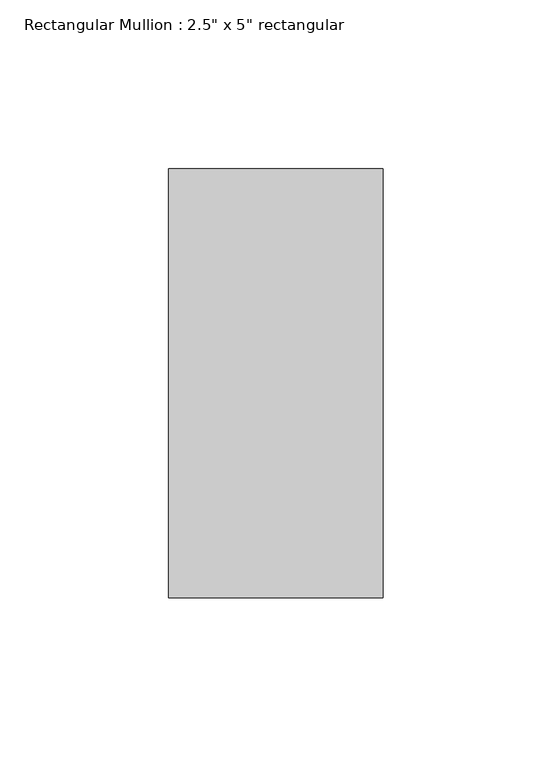
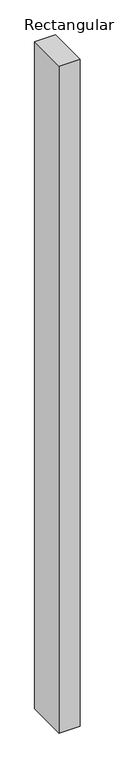
"""IFC4 building model written with IfcOpenShell, lengths in millimetres: member geometry."""

from ifc_helpers import new_model, si_unit, frame, origin, place, context, project, spatial, polyline, outline, extrude, source, transform, mapped, element, save


def member_cad56782(model_context):
    return source(origin(), model_context, "Body", "SweptSolid", [
        extrude(outline(polyline([(31.75, 63.5), (31.75, -63.5), (-31.75, -63.5), (-31.75, 63.5), (31.75, 63.5)])), frame((0.0, 0.0, -2129.1310998), z_axis=(0.0, 0.0, 1.0), x_axis=(1.0, 0.0, 0.0)), (0.0, 0.0, 1.0), 2129.1310998),
    ])


if __name__ == "__main__":
    model = new_model("IFC4")
    model_context = context("Model", 3, world=origin())
    ifc_project = project(units=[si_unit("LENGTHUNIT", "METRE", prefix="MILLI")], contexts=[model_context])
    site = spatial("IfcSite", under=ifc_project)
    building = spatial("IfcBuilding", under=site)
    placement = place(None, origin())
    member_shape = member_cad56782(model_context)
    element("IfcMember", 1, ObjectType="Rectangular Mullion : 2.5\" x 5\" rectangular", at=placement, inside=building, context=model_context, shape_type="MappedRepresentation", body=[
        mapped(member_shape, transform((0.0, 0.0, 0.0), x_axis=(1.0, 0.0, 0.0), y_axis=(0.0, 1.0, 0.0), z_axis=(0.0, 0.0, 1.0))),
    ])
    save(model, "model.ifc")

# Revit data of these elements
# Type "Rectangular Mullion : 2.5\" x 5\" rectangular"
#   built-in parameter 1007304 = 0.416667 (stored number, unit not read)
#   built-in parameter 1007301 = 0.104167 (stored number, unit not read)
#   built-in parameter 1007300 = 0.104167 (stored number, unit not read)
# Element 1 (IfcMember, "Rectangular Mullion : 2.5\" x 5\" rectangular")
#   Materials on its faces: "Aluminum"
# Materials
#   "Aluminum": class "Metal", colour RGB 247 247 247, transparency 0, Description = "Aluminum 6061", Cost = 0
